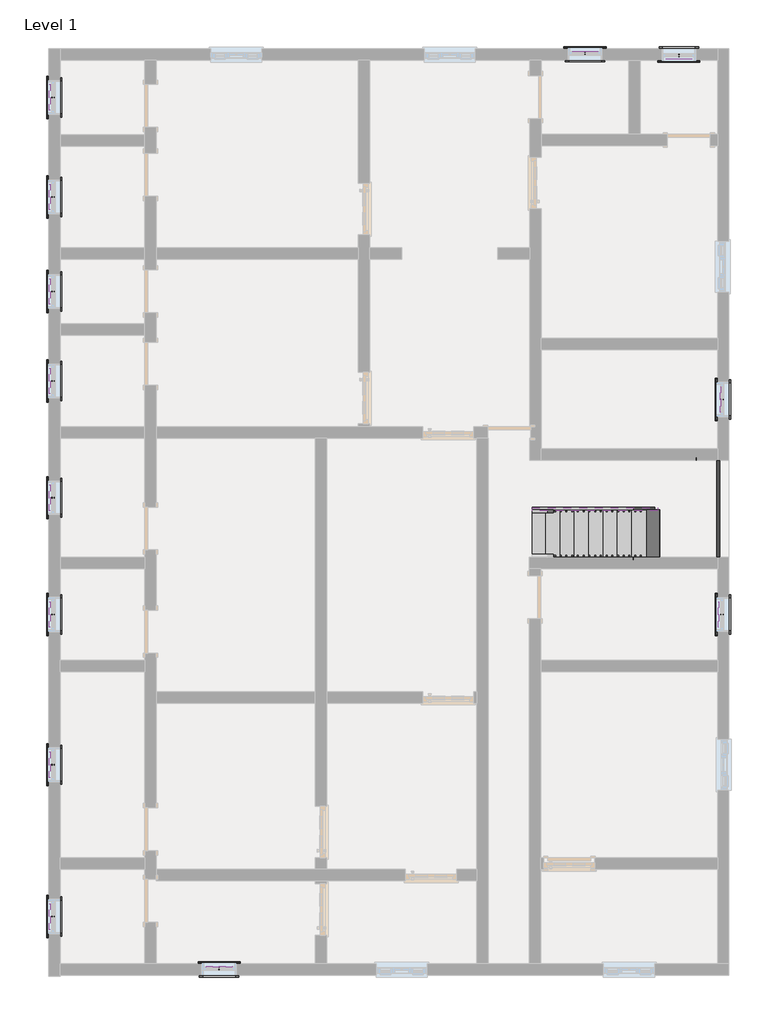
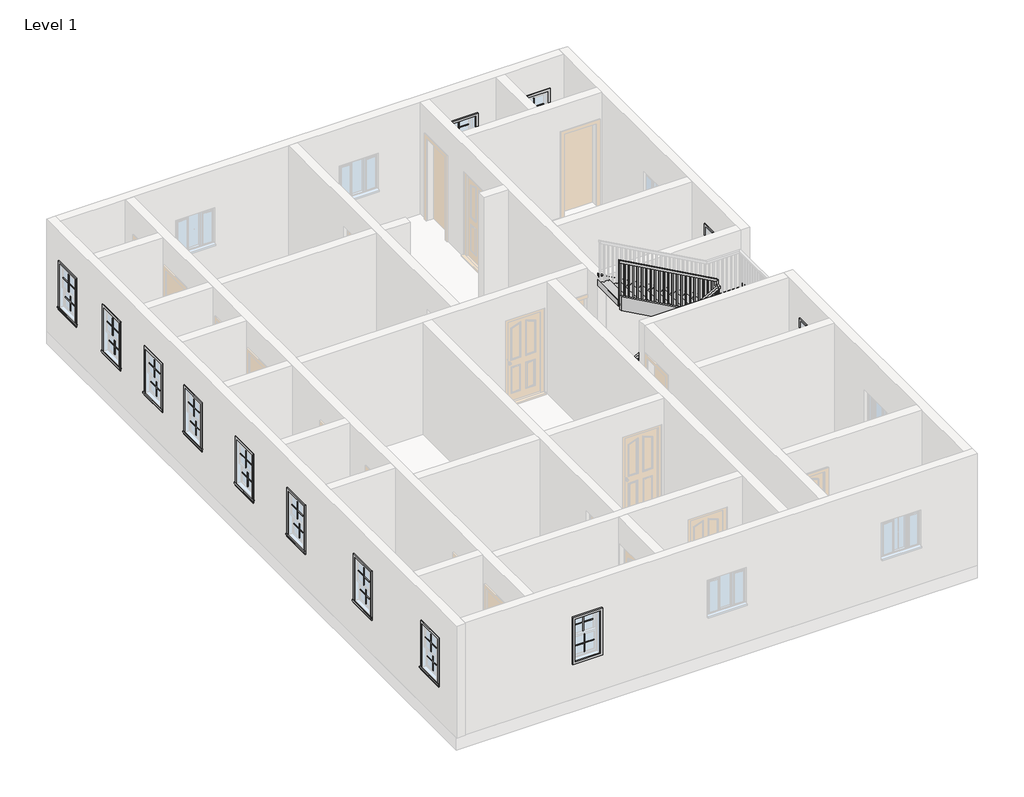
# One storey, part 3 of 3: 52 proxies, 5 members, 1 railing, 1 stair flight.
"""IFC4 building model written with IfcOpenShell, lengths in millimetres."""

from ifc_helpers import new_model, si_unit, frame, origin, place, context, project, spatial, polyline, outline, extrude, faceted_brep, transform, mapped, element, save
from components import muntin_pattern_2x2_muntin_pattern_2x2_eba6c5fb, trim_window_exterior_flat_with_sill_278e6a94, trim_window_interior_flat_picture_frame_e9fd5f45, stair_flight_18d05731

model = new_model("IFC4")

# Units and contexts
model_context = context("Model", 3, world=origin())
ifc_project = project(units=[si_unit("LENGTHUNIT", "METRE", prefix="MILLI")], contexts=[model_context])

# Site, building, storey
site = spatial("IfcSite", under=ifc_project)
building = spatial("IfcBuilding", under=site)
storey = spatial("IfcBuildingStorey", under=building, Name="Level 1", Elevation=0.0)

# Proxies
placement = place(None, origin())
muntin_pattern_2x2_muntin_pattern_2x2_shape = muntin_pattern_2x2_muntin_pattern_2x2_eba6c5fb(model_context)
element("IfcBuildingElementProxy", 1, Name="Muntin Pattern_2x2 : Muntin Pattern_2x2", ObjectType="Muntin Pattern_2x2 : Muntin Pattern_2x2", at=placement, inside=storey, context=model_context, shape_type="MappedRepresentation", body=[
    mapped(muntin_pattern_2x2_muntin_pattern_2x2_shape, transform((-10440.7626145, 6547.3404944, 1470.025), x_axis=(0.0, 1.0, 0.0), y_axis=(-1.0, 0.0, 0.0), z_axis=(0.0, 0.0, 1.0))),
])
element("IfcBuildingElementProxy", 2, Name="Muntin Pattern_2x2 : Muntin Pattern_2x2", ObjectType="Muntin Pattern_2x2 : Muntin Pattern_2x2", at=placement, inside=storey, context=model_context, shape_type="MappedRepresentation", body=[
    mapped(muntin_pattern_2x2_muntin_pattern_2x2_shape, transform((-10396.3126145, 6547.3404944, 990.6), x_axis=(0.0, 1.0, 0.0), y_axis=(-1.0, 0.0, 0.0), z_axis=(0.0, 0.0, 1.0))),
])
element("IfcBuildingElementProxy", 3, Name="Muntin Pattern_2x2 : Muntin Pattern_2x2", ObjectType="Muntin Pattern_2x2 : Muntin Pattern_2x2", at=placement, inside=storey, context=model_context, shape_type="MappedRepresentation", body=[
    mapped(muntin_pattern_2x2_muntin_pattern_2x2_shape, transform((-10440.7626145, 4782.0404944, 1470.025), x_axis=(0.0, 1.0, 0.0), y_axis=(-1.0, 0.0, 0.0), z_axis=(0.0, 0.0, 1.0))),
])
element("IfcBuildingElementProxy", 4, Name="Muntin Pattern_2x2 : Muntin Pattern_2x2", ObjectType="Muntin Pattern_2x2 : Muntin Pattern_2x2", at=placement, inside=storey, context=model_context, shape_type="MappedRepresentation", body=[
    mapped(muntin_pattern_2x2_muntin_pattern_2x2_shape, transform((-10396.3126145, 4782.0404944, 990.6), x_axis=(0.0, 1.0, 0.0), y_axis=(-1.0, 0.0, 0.0), z_axis=(0.0, 0.0, 1.0))),
])
element("IfcBuildingElementProxy", 5, Name="Muntin Pattern_2x2 : Muntin Pattern_2x2", ObjectType="Muntin Pattern_2x2 : Muntin Pattern_2x2", at=placement, inside=storey, context=model_context, shape_type="MappedRepresentation", body=[
    mapped(muntin_pattern_2x2_muntin_pattern_2x2_shape, transform((-10440.7626145, 3105.6404944, 1470.025), x_axis=(0.0, 1.0, 0.0), y_axis=(-1.0, 0.0, 0.0), z_axis=(0.0, 0.0, 1.0))),
])
element("IfcBuildingElementProxy", 6, Name="Muntin Pattern_2x2 : Muntin Pattern_2x2", ObjectType="Muntin Pattern_2x2 : Muntin Pattern_2x2", at=placement, inside=storey, context=model_context, shape_type="MappedRepresentation", body=[
    mapped(muntin_pattern_2x2_muntin_pattern_2x2_shape, transform((-10396.3126145, 3105.6404944, 990.6), x_axis=(0.0, 1.0, 0.0), y_axis=(-1.0, 0.0, 0.0), z_axis=(0.0, 0.0, 1.0))),
])
element("IfcBuildingElementProxy", 7, Name="Muntin Pattern_2x2 : Muntin Pattern_2x2", ObjectType="Muntin Pattern_2x2 : Muntin Pattern_2x2", at=placement, inside=storey, context=model_context, shape_type="MappedRepresentation", body=[
    mapped(muntin_pattern_2x2_muntin_pattern_2x2_shape, transform((-10440.7626145, 1518.1404944, 1470.025), x_axis=(0.0, 1.0, 0.0), y_axis=(-1.0, 0.0, 0.0), z_axis=(0.0, 0.0, 1.0))),
])
element("IfcBuildingElementProxy", 8, Name="Muntin Pattern_2x2 : Muntin Pattern_2x2", ObjectType="Muntin Pattern_2x2 : Muntin Pattern_2x2", at=placement, inside=storey, context=model_context, shape_type="MappedRepresentation", body=[
    mapped(muntin_pattern_2x2_muntin_pattern_2x2_shape, transform((-10396.3126145, 1518.1404944, 990.6), x_axis=(0.0, 1.0, 0.0), y_axis=(-1.0, 0.0, 0.0), z_axis=(0.0, 0.0, 1.0))),
])
element("IfcBuildingElementProxy", 9, Name="Muntin Pattern_2x2 : Muntin Pattern_2x2", ObjectType="Muntin Pattern_2x2 : Muntin Pattern_2x2", at=placement, inside=storey, context=model_context, shape_type="MappedRepresentation", body=[
    mapped(muntin_pattern_2x2_muntin_pattern_2x2_shape, transform((-10440.7626145, -551.9595056, 1470.025), x_axis=(0.0, 1.0, 0.0), y_axis=(-1.0, 0.0, 0.0), z_axis=(0.0, 0.0, 1.0))),
])
element("IfcBuildingElementProxy", 10, Name="Muntin Pattern_2x2 : Muntin Pattern_2x2", ObjectType="Muntin Pattern_2x2 : Muntin Pattern_2x2", at=placement, inside=storey, context=model_context, shape_type="MappedRepresentation", body=[
    mapped(muntin_pattern_2x2_muntin_pattern_2x2_shape, transform((-10396.3126145, -551.9595056, 990.6), x_axis=(0.0, 1.0, 0.0), y_axis=(-1.0, 0.0, 0.0), z_axis=(0.0, 0.0, 1.0))),
])
element("IfcBuildingElementProxy", 11, Name="Muntin Pattern_2x2 : Muntin Pattern_2x2", ObjectType="Muntin Pattern_2x2 : Muntin Pattern_2x2", at=placement, inside=storey, context=model_context, shape_type="MappedRepresentation", body=[
    mapped(muntin_pattern_2x2_muntin_pattern_2x2_shape, transform((-10440.7626145, -2622.0595056, 1470.025), x_axis=(0.0, 1.0, 0.0), y_axis=(-1.0, 0.0, 0.0), z_axis=(0.0, 0.0, 1.0))),
])
element("IfcBuildingElementProxy", 12, Name="Muntin Pattern_2x2 : Muntin Pattern_2x2", ObjectType="Muntin Pattern_2x2 : Muntin Pattern_2x2", at=placement, inside=storey, context=model_context, shape_type="MappedRepresentation", body=[
    mapped(muntin_pattern_2x2_muntin_pattern_2x2_shape, transform((-10396.3126145, -2622.0595056, 990.6), x_axis=(0.0, 1.0, 0.0), y_axis=(-1.0, 0.0, 0.0), z_axis=(0.0, 0.0, 1.0))),
])
element("IfcBuildingElementProxy", 13, Name="Muntin Pattern_2x2 : Muntin Pattern_2x2", ObjectType="Muntin Pattern_2x2 : Muntin Pattern_2x2", at=placement, inside=storey, context=model_context, shape_type="MappedRepresentation", body=[
    mapped(muntin_pattern_2x2_muntin_pattern_2x2_shape, transform((-10440.7626145, -5289.0595056, 1470.025), x_axis=(0.0, 1.0, 0.0), y_axis=(-1.0, 0.0, 0.0), z_axis=(0.0, 0.0, 1.0))),
])
element("IfcBuildingElementProxy", 14, Name="Muntin Pattern_2x2 : Muntin Pattern_2x2", ObjectType="Muntin Pattern_2x2 : Muntin Pattern_2x2", at=placement, inside=storey, context=model_context, shape_type="MappedRepresentation", body=[
    mapped(muntin_pattern_2x2_muntin_pattern_2x2_shape, transform((-10396.3126145, -5289.0595056, 990.6), x_axis=(0.0, 1.0, 0.0), y_axis=(-1.0, 0.0, 0.0), z_axis=(0.0, 0.0, 1.0))),
])
element("IfcBuildingElementProxy", 15, Name="Muntin Pattern_2x2 : Muntin Pattern_2x2", ObjectType="Muntin Pattern_2x2 : Muntin Pattern_2x2", at=placement, inside=storey, context=model_context, shape_type="MappedRepresentation", body=[
    mapped(muntin_pattern_2x2_muntin_pattern_2x2_shape, transform((-10440.7626145, -7981.4595056, 1470.025), x_axis=(0.0, 1.0, 0.0), y_axis=(-1.0, 0.0, 0.0), z_axis=(0.0, 0.0, 1.0))),
])
element("IfcBuildingElementProxy", 16, Name="Muntin Pattern_2x2 : Muntin Pattern_2x2", ObjectType="Muntin Pattern_2x2 : Muntin Pattern_2x2", at=placement, inside=storey, context=model_context, shape_type="MappedRepresentation", body=[
    mapped(muntin_pattern_2x2_muntin_pattern_2x2_shape, transform((-10396.3126145, -7981.4595056, 990.6), x_axis=(0.0, 1.0, 0.0), y_axis=(-1.0, 0.0, 0.0), z_axis=(0.0, 0.0, 1.0))),
])
element("IfcBuildingElementProxy", 17, Name="Muntin Pattern_2x2 : Muntin Pattern_2x2", ObjectType="Muntin Pattern_2x2 : Muntin Pattern_2x2", at=placement, inside=storey, context=model_context, shape_type="MappedRepresentation", body=[
    mapped(muntin_pattern_2x2_muntin_pattern_2x2_shape, transform((-7453.0876145, -8854.5845056, 1470.025), x_axis=(1.0, 0.0, 0.0), y_axis=(0.0, 1.0, 0.0), z_axis=(0.0, 0.0, 1.0))),
])
element("IfcBuildingElementProxy", 18, Name="Muntin Pattern_2x2 : Muntin Pattern_2x2", ObjectType="Muntin Pattern_2x2 : Muntin Pattern_2x2", at=placement, inside=storey, context=model_context, shape_type="MappedRepresentation", body=[
    mapped(muntin_pattern_2x2_muntin_pattern_2x2_shape, transform((-7453.0876145, -8899.0345056, 990.6), x_axis=(1.0, 0.0, 0.0), y_axis=(0.0, 1.0, 0.0), z_axis=(0.0, 0.0, 1.0))),
])
element("IfcBuildingElementProxy", 19, Name="Muntin Pattern_2x2 : Muntin Pattern_2x2", ObjectType="Muntin Pattern_2x2 : Muntin Pattern_2x2", at=placement, inside=storey, context=model_context, shape_type="MappedRepresentation", body=[
    mapped(muntin_pattern_2x2_muntin_pattern_2x2_shape, transform((1421.0373855, -2622.0595056, 1470.025), x_axis=(0.0, 1.0, 0.0), y_axis=(-1.0, 0.0, 0.0), z_axis=(0.0, 0.0, 1.0))),
])
element("IfcBuildingElementProxy", 20, Name="Muntin Pattern_2x2 : Muntin Pattern_2x2", ObjectType="Muntin Pattern_2x2 : Muntin Pattern_2x2", at=placement, inside=storey, context=model_context, shape_type="MappedRepresentation", body=[
    mapped(muntin_pattern_2x2_muntin_pattern_2x2_shape, transform((1465.4873855, -2622.0595056, 990.6), x_axis=(0.0, 1.0, 0.0), y_axis=(-1.0, 0.0, 0.0), z_axis=(0.0, 0.0, 1.0))),
])
element("IfcBuildingElementProxy", 21, Name="Muntin Pattern_2x2 : Muntin Pattern_2x2", ObjectType="Muntin Pattern_2x2 : Muntin Pattern_2x2", at=placement, inside=storey, context=model_context, shape_type="MappedRepresentation", body=[
    mapped(muntin_pattern_2x2_muntin_pattern_2x2_shape, transform((1421.0373855, 1190.4645364, 1470.025), x_axis=(0.0, 1.0, 0.0), y_axis=(-1.0, 0.0, 0.0), z_axis=(0.0, 0.0, 1.0))),
])
element("IfcBuildingElementProxy", 22, Name="Muntin Pattern_2x2 : Muntin Pattern_2x2", ObjectType="Muntin Pattern_2x2 : Muntin Pattern_2x2", at=placement, inside=storey, context=model_context, shape_type="MappedRepresentation", body=[
    mapped(muntin_pattern_2x2_muntin_pattern_2x2_shape, transform((1465.4873855, 1190.4645364, 990.6), x_axis=(0.0, 1.0, 0.0), y_axis=(-1.0, 0.0, 0.0), z_axis=(0.0, 0.0, 1.0))),
])
element("IfcBuildingElementProxy", 23, Name="Muntin Pattern_2x2 : Muntin Pattern_2x2", ObjectType="Muntin Pattern_2x2 : Muntin Pattern_2x2", at=placement, inside=storey, context=model_context, shape_type="MappedRepresentation", body=[
    mapped(muntin_pattern_2x2_muntin_pattern_2x2_shape, transform((700.3123855, 7242.6654944, 1470.025), x_axis=(-1.0, 0.0, 0.0), y_axis=(0.0, -1.0, 0.0), z_axis=(0.0, 0.0, 1.0))),
])
element("IfcBuildingElementProxy", 24, Name="Muntin Pattern_2x2 : Muntin Pattern_2x2", ObjectType="Muntin Pattern_2x2 : Muntin Pattern_2x2", at=placement, inside=storey, context=model_context, shape_type="MappedRepresentation", body=[
    mapped(muntin_pattern_2x2_muntin_pattern_2x2_shape, transform((700.3123855, 7287.1154944, 990.6), x_axis=(-1.0, 0.0, 0.0), y_axis=(0.0, -1.0, 0.0), z_axis=(0.0, 0.0, 1.0))),
])
element("IfcBuildingElementProxy", 25, Name="Muntin Pattern_2x2 : Muntin Pattern_2x2", ObjectType="Muntin Pattern_2x2 : Muntin Pattern_2x2", at=placement, inside=storey, context=model_context, shape_type="MappedRepresentation", body=[
    mapped(muntin_pattern_2x2_muntin_pattern_2x2_shape, transform((-963.3876145, 7376.0154944, 1470.025), x_axis=(1.0, 0.0, 0.0), y_axis=(0.0, 1.0, 0.0), z_axis=(0.0, 0.0, 1.0))),
])
element("IfcBuildingElementProxy", 26, Name="Muntin Pattern_2x2 : Muntin Pattern_2x2", ObjectType="Muntin Pattern_2x2 : Muntin Pattern_2x2", at=placement, inside=storey, context=model_context, shape_type="MappedRepresentation", body=[
    mapped(muntin_pattern_2x2_muntin_pattern_2x2_shape, transform((-963.3876145, 7331.5654944, 990.6), x_axis=(1.0, 0.0, 0.0), y_axis=(0.0, 1.0, 0.0), z_axis=(0.0, 0.0, 1.0))),
])
trim_window_exterior_flat_with_sill_shape = trim_window_exterior_flat_with_sill_278e6a94(model_context)
element("IfcBuildingElementProxy", 27, Name="Trim-Window-Exterior-Flat : with Sill", ObjectType="Trim-Window-Exterior-Flat : with Sill", at=placement, inside=storey, context=model_context, shape_type="MappedRepresentation", body=[
    mapped(trim_window_exterior_flat_with_sill_shape, transform((-10475.6876145, 6547.3404944, 1981.2), x_axis=(0.0, -1.0, 0.0), y_axis=(0.0, 0.0, 1.0), z_axis=(-1.0, 0.0, 0.0))),
])
element("IfcBuildingElementProxy", 28, Name="Trim-Window-Exterior-Flat : with Sill", ObjectType="Trim-Window-Exterior-Flat : with Sill", at=placement, inside=storey, context=model_context, shape_type="MappedRepresentation", body=[
    mapped(trim_window_exterior_flat_with_sill_shape, transform((-10475.6876145, 4782.0404944, 1981.2), x_axis=(0.0, -1.0, 0.0), y_axis=(0.0, 0.0, 1.0), z_axis=(-1.0, 0.0, 0.0))),
])
element("IfcBuildingElementProxy", 29, Name="Trim-Window-Exterior-Flat : with Sill", ObjectType="Trim-Window-Exterior-Flat : with Sill", at=placement, inside=storey, context=model_context, shape_type="MappedRepresentation", body=[
    mapped(trim_window_exterior_flat_with_sill_shape, transform((-10475.6876145, 3105.6404944, 1981.2), x_axis=(0.0, -1.0, 0.0), y_axis=(0.0, 0.0, 1.0), z_axis=(-1.0, 0.0, 0.0))),
])
element("IfcBuildingElementProxy", 30, Name="Trim-Window-Exterior-Flat : with Sill", ObjectType="Trim-Window-Exterior-Flat : with Sill", at=placement, inside=storey, context=model_context, shape_type="MappedRepresentation", body=[
    mapped(trim_window_exterior_flat_with_sill_shape, transform((-10475.6876145, 1518.1404944, 1981.2), x_axis=(0.0, -1.0, 0.0), y_axis=(0.0, 0.0, 1.0), z_axis=(-1.0, 0.0, 0.0))),
])
element("IfcBuildingElementProxy", 31, Name="Trim-Window-Exterior-Flat : with Sill", ObjectType="Trim-Window-Exterior-Flat : with Sill", at=placement, inside=storey, context=model_context, shape_type="MappedRepresentation", body=[
    mapped(trim_window_exterior_flat_with_sill_shape, transform((-10475.6876145, -551.9595056, 1981.2), x_axis=(0.0, -1.0, 0.0), y_axis=(0.0, 0.0, 1.0), z_axis=(-1.0, 0.0, 0.0))),
])
element("IfcBuildingElementProxy", 32, Name="Trim-Window-Exterior-Flat : with Sill", ObjectType="Trim-Window-Exterior-Flat : with Sill", at=placement, inside=storey, context=model_context, shape_type="MappedRepresentation", body=[
    mapped(trim_window_exterior_flat_with_sill_shape, transform((-10475.6876145, -2622.0595056, 1981.2), x_axis=(0.0, -1.0, 0.0), y_axis=(0.0, 0.0, 1.0), z_axis=(-1.0, 0.0, 0.0))),
])
element("IfcBuildingElementProxy", 33, Name="Trim-Window-Exterior-Flat : with Sill", ObjectType="Trim-Window-Exterior-Flat : with Sill", at=placement, inside=storey, context=model_context, shape_type="MappedRepresentation", body=[
    mapped(trim_window_exterior_flat_with_sill_shape, transform((-10475.6876145, -5289.0595056, 1981.2), x_axis=(0.0, -1.0, 0.0), y_axis=(0.0, 0.0, 1.0), z_axis=(-1.0, 0.0, 0.0))),
])
element("IfcBuildingElementProxy", 34, Name="Trim-Window-Exterior-Flat : with Sill", ObjectType="Trim-Window-Exterior-Flat : with Sill", at=placement, inside=storey, context=model_context, shape_type="MappedRepresentation", body=[
    mapped(trim_window_exterior_flat_with_sill_shape, transform((-10475.6876145, -7981.4595056, 1981.2), x_axis=(0.0, -1.0, 0.0), y_axis=(0.0, 0.0, 1.0), z_axis=(-1.0, 0.0, 0.0))),
])
element("IfcBuildingElementProxy", 35, Name="Trim-Window-Exterior-Flat : with Sill", ObjectType="Trim-Window-Exterior-Flat : with Sill", at=placement, inside=storey, context=model_context, shape_type="MappedRepresentation", body=[
    mapped(trim_window_exterior_flat_with_sill_shape, transform((-7453.0876145, -8819.6595056, 1981.2), x_axis=(-1.0, 0.0, 0.0), y_axis=(0.0, 0.0, 1.0), z_axis=(0.0, 1.0, 0.0))),
])
element("IfcBuildingElementProxy", 36, Name="Trim-Window-Exterior-Flat : with Sill", ObjectType="Trim-Window-Exterior-Flat : with Sill", at=placement, inside=storey, context=model_context, shape_type="MappedRepresentation", body=[
    mapped(trim_window_exterior_flat_with_sill_shape, transform((1386.1123855, -2622.0595056, 1981.2), x_axis=(0.0, -1.0, 0.0), y_axis=(0.0, 0.0, 1.0), z_axis=(-1.0, 0.0, 0.0))),
])
element("IfcBuildingElementProxy", 37, Name="Trim-Window-Exterior-Flat : with Sill", ObjectType="Trim-Window-Exterior-Flat : with Sill", at=placement, inside=storey, context=model_context, shape_type="MappedRepresentation", body=[
    mapped(trim_window_exterior_flat_with_sill_shape, transform((1386.1123855, 1190.4645364, 1981.2), x_axis=(0.0, -1.0, 0.0), y_axis=(0.0, 0.0, 1.0), z_axis=(-1.0, 0.0, 0.0))),
])
element("IfcBuildingElementProxy", 38, Name="Trim-Window-Exterior-Flat : with Sill", ObjectType="Trim-Window-Exterior-Flat : with Sill", at=placement, inside=storey, context=model_context, shape_type="MappedRepresentation", body=[
    mapped(trim_window_exterior_flat_with_sill_shape, transform((700.3123855, 7207.7404944, 1981.2), x_axis=(1.0, 0.0, 0.0), y_axis=(0.0, 0.0, 1.0), z_axis=(0.0, -1.0, 0.0))),
])
element("IfcBuildingElementProxy", 39, Name="Trim-Window-Exterior-Flat : with Sill", ObjectType="Trim-Window-Exterior-Flat : with Sill", at=placement, inside=storey, context=model_context, shape_type="MappedRepresentation", body=[
    mapped(trim_window_exterior_flat_with_sill_shape, transform((-963.3876145, 7410.9404944, 1981.2), x_axis=(-1.0, 0.0, 0.0), y_axis=(0.0, 0.0, 1.0), z_axis=(0.0, 1.0, 0.0))),
])
trim_window_interior_flat_picture_frame_shape = trim_window_interior_flat_picture_frame_e9fd5f45(model_context)
element("IfcBuildingElementProxy", 40, Name="Trim-Window-Interior-Flat : Picture Frame", ObjectType="Trim-Window-Interior-Flat : Picture Frame", at=placement, inside=storey, context=model_context, shape_type="MappedRepresentation", body=[
    mapped(trim_window_interior_flat_picture_frame_shape, transform((-10272.4876145, 6547.3404944, 1981.2), x_axis=(0.0, 1.0, 0.0), y_axis=(0.0, 0.0, 1.0), z_axis=(1.0, 0.0, 0.0))),
])
element("IfcBuildingElementProxy", 41, Name="Trim-Window-Interior-Flat : Picture Frame", ObjectType="Trim-Window-Interior-Flat : Picture Frame", at=placement, inside=storey, context=model_context, shape_type="MappedRepresentation", body=[
    mapped(trim_window_interior_flat_picture_frame_shape, transform((-10272.4876145, 4782.0404944, 1981.2), x_axis=(0.0, 1.0, 0.0), y_axis=(0.0, 0.0, 1.0), z_axis=(1.0, 0.0, 0.0))),
])
element("IfcBuildingElementProxy", 42, Name="Trim-Window-Interior-Flat : Picture Frame", ObjectType="Trim-Window-Interior-Flat : Picture Frame", at=placement, inside=storey, context=model_context, shape_type="MappedRepresentation", body=[
    mapped(trim_window_interior_flat_picture_frame_shape, transform((-10272.4876145, 3105.6404944, 1981.2), x_axis=(0.0, 1.0, 0.0), y_axis=(0.0, 0.0, 1.0), z_axis=(1.0, 0.0, 0.0))),
])
element("IfcBuildingElementProxy", 43, Name="Trim-Window-Interior-Flat : Picture Frame", ObjectType="Trim-Window-Interior-Flat : Picture Frame", at=placement, inside=storey, context=model_context, shape_type="MappedRepresentation", body=[
    mapped(trim_window_interior_flat_picture_frame_shape, transform((-10272.4876145, 1518.1404944, 1981.2), x_axis=(0.0, 1.0, 0.0), y_axis=(0.0, 0.0, 1.0), z_axis=(1.0, 0.0, 0.0))),
])
element("IfcBuildingElementProxy", 44, Name="Trim-Window-Interior-Flat : Picture Frame", ObjectType="Trim-Window-Interior-Flat : Picture Frame", at=placement, inside=storey, context=model_context, shape_type="MappedRepresentation", body=[
    mapped(trim_window_interior_flat_picture_frame_shape, transform((-10272.4876145, -551.9595056, 1981.2), x_axis=(0.0, 1.0, 0.0), y_axis=(0.0, 0.0, 1.0), z_axis=(1.0, 0.0, 0.0))),
])
element("IfcBuildingElementProxy", 45, Name="Trim-Window-Interior-Flat : Picture Frame", ObjectType="Trim-Window-Interior-Flat : Picture Frame", at=placement, inside=storey, context=model_context, shape_type="MappedRepresentation", body=[
    mapped(trim_window_interior_flat_picture_frame_shape, transform((-10272.4876145, -2622.0595056, 1981.2), x_axis=(0.0, 1.0, 0.0), y_axis=(0.0, 0.0, 1.0), z_axis=(1.0, 0.0, 0.0))),
])
element("IfcBuildingElementProxy", 46, Name="Trim-Window-Interior-Flat : Picture Frame", ObjectType="Trim-Window-Interior-Flat : Picture Frame", at=placement, inside=storey, context=model_context, shape_type="MappedRepresentation", body=[
    mapped(trim_window_interior_flat_picture_frame_shape, transform((-10272.4876145, -5289.0595056, 1981.2), x_axis=(0.0, 1.0, 0.0), y_axis=(0.0, 0.0, 1.0), z_axis=(1.0, 0.0, 0.0))),
])
element("IfcBuildingElementProxy", 47, Name="Trim-Window-Interior-Flat : Picture Frame", ObjectType="Trim-Window-Interior-Flat : Picture Frame", at=placement, inside=storey, context=model_context, shape_type="MappedRepresentation", body=[
    mapped(trim_window_interior_flat_picture_frame_shape, transform((-10272.4876145, -7981.4595056, 1981.2), x_axis=(0.0, 1.0, 0.0), y_axis=(0.0, 0.0, 1.0), z_axis=(1.0, 0.0, 0.0))),
])
element("IfcBuildingElementProxy", 48, Name="Trim-Window-Interior-Flat : Picture Frame", ObjectType="Trim-Window-Interior-Flat : Picture Frame", at=placement, inside=storey, context=model_context, shape_type="MappedRepresentation", body=[
    mapped(trim_window_interior_flat_picture_frame_shape, transform((-7453.0876145, -9022.8595056, 1981.2), x_axis=(1.0, 0.0, 0.0), y_axis=(0.0, 0.0, 1.0), z_axis=(0.0, -1.0, 0.0))),
])
element("IfcBuildingElementProxy", 49, Name="Trim-Window-Interior-Flat : Picture Frame", ObjectType="Trim-Window-Interior-Flat : Picture Frame", at=placement, inside=storey, context=model_context, shape_type="MappedRepresentation", body=[
    mapped(trim_window_interior_flat_picture_frame_shape, transform((1589.3123855, -2622.0595056, 1981.2), x_axis=(0.0, 1.0, 0.0), y_axis=(0.0, 0.0, 1.0), z_axis=(1.0, 0.0, 0.0))),
])
element("IfcBuildingElementProxy", 50, Name="Trim-Window-Interior-Flat : Picture Frame", ObjectType="Trim-Window-Interior-Flat : Picture Frame", at=placement, inside=storey, context=model_context, shape_type="MappedRepresentation", body=[
    mapped(trim_window_interior_flat_picture_frame_shape, transform((1589.3123855, 1190.4645364, 1981.2), x_axis=(0.0, 1.0, 0.0), y_axis=(0.0, 0.0, 1.0), z_axis=(1.0, 0.0, 0.0))),
])
element("IfcBuildingElementProxy", 51, Name="Trim-Window-Interior-Flat : Picture Frame", ObjectType="Trim-Window-Interior-Flat : Picture Frame", at=placement, inside=storey, context=model_context, shape_type="MappedRepresentation", body=[
    mapped(trim_window_interior_flat_picture_frame_shape, transform((700.3123855, 7410.9404944, 1981.2), x_axis=(-1.0, 0.0, 0.0), y_axis=(0.0, 0.0, 1.0), z_axis=(0.0, 1.0, 0.0))),
])
element("IfcBuildingElementProxy", 52, Name="Trim-Window-Interior-Flat : Picture Frame", ObjectType="Trim-Window-Interior-Flat : Picture Frame", at=placement, inside=storey, context=model_context, shape_type="MappedRepresentation", body=[
    mapped(trim_window_interior_flat_picture_frame_shape, transform((-963.3876145, 7207.7404944, 1981.2), x_axis=(1.0, 0.0, 0.0), y_axis=(0.0, 0.0, 1.0), z_axis=(0.0, -1.0, 0.0))),
])

# Members
element("IfcMember", 53, ObjectType="Stringer - 2\" Width", at=placement, inside=storey, context=model_context, shape_type="SweptSolid", body=[
    extrude(outline(polyline([(210.6757607, -1903.1876145), (0.0, -1903.1876145), (0.0, -1654.2050647), (1065.4963497, 274.6830625), (1413.7073019, 274.6830625), (210.6757607, -1903.1876145)])), frame((0.0, -767.8595056, 0.0), z_axis=(0.0, 1.0, 0.0), x_axis=(0.0, 0.0, 1.0)), (0.0, 0.0, 1.0), 50.8),
])
element("IfcMember", 54, ObjectType="Stringer - 2\" Width", at=placement, inside=storey, context=model_context, shape_type="SweptSolid", body=[
    extrude(outline(polyline([(1230.7177047, 325.4830625), (1578.928657, 325.4830625), (2810.0215532, -1903.1876145), (2461.8106009, -1903.1876145), (1230.7177047, 325.4830625)])), frame((0.0, -780.5595056, 0.0), z_axis=(0.0, 1.0, 0.0), x_axis=(0.0, 0.0, 1.0)), (0.0, 0.0, 1.0), 50.8),
])
element("IfcMember", 55, ObjectType="Stringer - 2\" Width", at=placement, inside=storey, context=model_context, shape_type="SweptSolid", body=[
    extrude(outline(polyline([(210.6757607, -1903.1876145), (0.0, -1903.1876145), (0.0, -1654.2050647), (1447.8, 966.7745674), (1447.8, 336.4017165), (210.6757607, -1903.1876145)])), frame((0.0, -1656.8595056, 0.0), z_axis=(0.0, 1.0, 0.0), x_axis=(0.0, 0.0, 1.0)), (0.0, 0.0, 1.0), 50.8),
])
element("IfcMember", 56, ObjectType="Stringer - 2\" Width", at=placement, inside=storey, context=model_context, shape_type="SweptSolid", body=[
    extrude(outline(polyline([(1424.2123855, -1656.8595056), (1373.4123855, -1656.8595056), (1373.4123855, 108.4404944), (1424.2123855, 108.4404944), (1424.2123855, -1656.8595056)])), frame((0.0, 0.0, 1143.0), z_axis=(0.0, 0.0, 1.0), x_axis=(1.0, 0.0, 0.0)), (0.0, 0.0, 1.0), 304.8),
])
element("IfcMember", 57, ObjectType="Stringer - 2\" Width", at=placement, inside=storey, context=model_context, shape_type="SweptSolid", body=[
    extrude(outline(polyline([(1143.0, 1114.6529278), (2810.0215532, -1903.1876145), (2461.8106009, -1903.1876145), (1143.0, 484.2800769), (1143.0, 1114.6529278)])), frame((0.0, 108.4404944, 0.0), z_axis=(0.0, 1.0, 0.0), x_axis=(0.0, 0.0, 1.0)), (0.0, 0.0, 1.0), 50.8),
])

# Railing
element("IfcRailing", 58, ObjectType="Handrail - Rectangular", at=placement, inside=storey, context=model_context, shape_type="SolidModel", body=[
    faceted_brep([(-1903.1876145, -767.8595056, 1051.56), (-1903.1876145, -767.8595056, 993.4879132), (-1903.1876145, -818.6595056, 993.4879132), (-1903.1876145, -818.6595056, 1051.56), (325.4830625, -767.8595056, 2286.0), (325.4830625, -818.6595056, 2286.0), (325.4830625, -818.6595056, 2227.9279132), (325.4830625, -767.8595056, 2227.9279132)], [[[0, 1, 2, 3]], [[4, 5, 6, 7]], [[1, 0, 4, 7]], [[2, 1, 7, 6]], [[3, 2, 6, 5]], [[0, 3, 5, 4]]]),
    faceted_brep([(325.4830625, -818.6595056, 2286.0), (325.4830625, -818.6595056, 2235.2), (376.2830625, -818.6595056, 2235.2), (376.2830625, -818.6595056, 2286.0), (325.4830625, -729.7595056, 2286.0), (376.2830625, -729.7595056, 2286.0), (376.2830625, -678.9595056, 2235.2), (325.4830625, -678.9595056, 2235.2)], [[[0, 1, 2, 3]], [[4, 5, 6, 7]], [[1, 0, 4, 7]], [[2, 1, 7, 6]], [[3, 2, 6, 5]], [[0, 3, 5, 4]]]),
    faceted_brep([(325.4830625, -729.7595056, 2286.0), (325.4830625, -678.9595056, 2235.2), (376.2830625, -678.9595056, 2235.2), (376.2830625, -729.7595056, 2286.0), (325.4830625, -729.7595056, 2365.0879132), (376.2830625, -729.7595056, 2395.0223516), (376.2830625, -678.9595056, 2395.0223516), (325.4830625, -678.9595056, 2365.0879132)], [[[0, 1, 2, 3]], [[4, 5, 6, 7]], [[1, 0, 4, 7]], [[2, 1, 7, 6]], [[3, 2, 6, 5]], [[0, 3, 5, 4]]]),
    faceted_brep([(376.2830625, -729.7595056, 2395.0223516), (325.4830625, -729.7595056, 2365.0879132), (325.4830625, -678.9595056, 2365.0879132), (376.2830625, -678.9595056, 2395.0223516), (-1903.1876145, -729.7595056, 3657.6), (-1903.1876145, -678.9595056, 3657.6), (-1903.1876145, -678.9595056, 3599.5279132), (-1903.1876145, -729.7595056, 3599.5279132)], [[[0, 1, 2, 3]], [[4, 5, 6, 7]], [[1, 0, 4, 7]], [[2, 1, 7, 6]], [[3, 2, 6, 5]], [[0, 3, 5, 4]]]),
    extrude(outline(polyline([(3594.3072849, -1893.8419375), (2606.04, -1893.8419375), (2606.04, -1874.7919375), (3583.7556667, -1874.7919375), (3594.3072849, -1893.8419375)])), frame((0.0, -713.8845056, 0.0), z_axis=(0.0, 1.0, 0.0), x_axis=(0.0, 0.0, 1.0)), (0.0, 0.0, 1.0), 19.05),
    extrude(outline(polyline([(3538.031988, -1792.2419375), (2606.04, -1792.2419375), (2606.04, -1773.1919375), (3527.4803699, -1773.1919375), (3538.031988, -1792.2419375)])), frame((0.0, -713.8845056, 0.0), z_axis=(0.0, 1.0, 0.0), x_axis=(0.0, 0.0, 1.0)), (0.0, 0.0, 1.0), 19.05),
    extrude(outline(polyline([(3481.7125466, -1690.6419375), (2606.04, -1690.6419375), (2606.04, -1671.5919375), (3471.1609284, -1671.5919375), (3481.7125466, -1690.6419375)])), frame((0.0, -713.8845056, 0.0), z_axis=(0.0, 1.0, 0.0), x_axis=(0.0, 0.0, 1.0)), (0.0, 0.0, 1.0), 19.05),
    extrude(outline(polyline([(3425.4813943, -1589.0419375), (2468.88, -1589.0419375), (2468.88, -1569.9919375), (3414.9297761, -1569.9919375), (3425.4813943, -1589.0419375)])), frame((0.0, -713.8845056, 0.0), z_axis=(0.0, 1.0, 0.0), x_axis=(0.0, 0.0, 1.0)), (0.0, 0.0, 1.0), 19.05),
    extrude(outline(polyline([(3369.2060974, -1487.4419375), (2468.88, -1487.4419375), (2468.88, -1468.3919375), (3358.6544792, -1468.3919375), (3369.2060974, -1487.4419375)])), frame((0.0, -713.8845056, 0.0), z_axis=(0.0, 1.0, 0.0), x_axis=(0.0, 0.0, 1.0)), (0.0, 0.0, 1.0), 19.05),
    extrude(outline(polyline([(3312.9308005, -1385.8419375), (2331.72, -1385.8419375), (2331.72, -1366.7919375), (3302.3791823, -1366.7919375), (3312.9308005, -1385.8419375)])), frame((0.0, -713.8845056, 0.0), z_axis=(0.0, 1.0, 0.0), x_axis=(0.0, 0.0, 1.0)), (0.0, 0.0, 1.0), 19.05),
    extrude(outline(polyline([(3256.6555036, -1284.2419375), (2331.72, -1284.2419375), (2331.72, -1265.1919375), (3246.1038855, -1265.1919375), (3256.6555036, -1284.2419375)])), frame((0.0, -713.8845056, 0.0), z_axis=(0.0, 1.0, 0.0), x_axis=(0.0, 0.0, 1.0)), (0.0, 0.0, 1.0), 19.05),
    extrude(outline(polyline([(3200.3802067, -1182.6419375), (2331.72, -1182.6419375), (2331.72, -1163.5919375), (3189.8285886, -1163.5919375), (3200.3802067, -1182.6419375)])), frame((0.0, -713.8845056, 0.0), z_axis=(0.0, 1.0, 0.0), x_axis=(0.0, 0.0, 1.0)), (0.0, 0.0, 1.0), 19.05),
    extrude(outline(polyline([(3144.1049099, -1081.0419375), (2194.56, -1081.0419375), (2194.56, -1061.9919375), (3133.5532917, -1061.9919375), (3144.1049099, -1081.0419375)])), frame((0.0, -713.8845056, 0.0), z_axis=(0.0, 1.0, 0.0), x_axis=(0.0, 0.0, 1.0)), (0.0, 0.0, 1.0), 19.05),
    extrude(outline(polyline([(3087.829613, -979.4419375), (2194.56, -979.4419375), (2194.56, -960.3919375), (3077.2779948, -960.3919375), (3087.829613, -979.4419375)])), frame((0.0, -713.8845056, 0.0), z_axis=(0.0, 1.0, 0.0), x_axis=(0.0, 0.0, 1.0)), (0.0, 0.0, 1.0), 19.05),
    extrude(outline(polyline([(3031.5543161, -877.8419375), (2057.4, -877.8419375), (2057.4, -858.7919375), (3021.0026979, -858.7919375), (3031.5543161, -877.8419375)])), frame((0.0, -713.8845056, 0.0), z_axis=(0.0, 1.0, 0.0), x_axis=(0.0, 0.0, 1.0)), (0.0, 0.0, 1.0), 19.05),
    extrude(outline(polyline([(2975.2790192, -776.2419375), (2057.4, -776.2419375), (2057.4, -757.1919375), (2964.727401, -757.1919375), (2975.2790192, -776.2419375)])), frame((0.0, -713.8845056, 0.0), z_axis=(0.0, 1.0, 0.0), x_axis=(0.0, 0.0, 1.0)), (0.0, 0.0, 1.0), 19.05),
    extrude(outline(polyline([(2919.0478669, -674.6419375), (2057.4, -674.6419375), (2057.4, -655.5919375), (2908.4962488, -655.5919375), (2919.0478669, -674.6419375)])), frame((0.0, -713.8845056, 0.0), z_axis=(0.0, 1.0, 0.0), x_axis=(0.0, 0.0, 1.0)), (0.0, 0.0, 1.0), 19.05),
    extrude(outline(polyline([(2862.77257, -573.0419375), (1920.24, -573.0419375), (1920.24, -553.9919375), (2852.2209519, -553.9919375), (2862.77257, -573.0419375)])), frame((0.0, -713.8845056, 0.0), z_axis=(0.0, 1.0, 0.0), x_axis=(0.0, 0.0, 1.0)), (0.0, 0.0, 1.0), 19.05),
    extrude(outline(polyline([(2806.4972732, -471.4419375), (1920.24, -471.4419375), (1920.24, -452.3919375), (2795.945655, -452.3919375), (2806.4972732, -471.4419375)])), frame((0.0, -713.8845056, 0.0), z_axis=(0.0, 1.0, 0.0), x_axis=(0.0, 0.0, 1.0)), (0.0, 0.0, 1.0), 19.05),
    extrude(outline(polyline([(2750.2219763, -369.8419375), (1783.08, -369.8419375), (1783.08, -350.7919375), (2739.6703581, -350.7919375), (2750.2219763, -369.8419375)])), frame((0.0, -713.8845056, 0.0), z_axis=(0.0, 1.0, 0.0), x_axis=(0.0, 0.0, 1.0)), (0.0, 0.0, 1.0), 19.05),
    extrude(outline(polyline([(2693.9466794, -268.2419375), (1783.08, -268.2419375), (1783.08, -249.1919375), (2683.3950612, -249.1919375), (2693.9466794, -268.2419375)])), frame((0.0, -713.8845056, 0.0), z_axis=(0.0, 1.0, 0.0), x_axis=(0.0, 0.0, 1.0)), (0.0, 0.0, 1.0), 19.05),
    extrude(outline(polyline([(2637.6713825, -166.6419375), (1783.08, -166.6419375), (1783.08, -147.5919375), (2627.1197643, -147.5919375), (2637.6713825, -166.6419375)])), frame((0.0, -713.8845056, 0.0), z_axis=(0.0, 1.0, 0.0), x_axis=(0.0, 0.0, 1.0)), (0.0, 0.0, 1.0), 19.05),
    extrude(outline(polyline([(2581.3960856, -65.0419375), (1645.92, -65.0419375), (1645.92, -45.9919375), (2570.8444675, -45.9919375), (2581.3960856, -65.0419375)])), frame((0.0, -713.8845056, 0.0), z_axis=(0.0, 1.0, 0.0), x_axis=(0.0, 0.0, 1.0)), (0.0, 0.0, 1.0), 19.05),
    extrude(outline(polyline([(2525.1207888, 36.5580625), (1645.92, 36.5580625), (1645.92, 55.6080625), (2514.5691706, 55.6080625), (2525.1207888, 36.5580625)])), frame((0.0, -713.8845056, 0.0), z_axis=(0.0, 1.0, 0.0), x_axis=(0.0, 0.0, 1.0)), (0.0, 0.0, 1.0), 19.05),
    extrude(outline(polyline([(2468.8454919, 138.1580625), (1508.76, 138.1580625), (1508.76, 157.2080625), (2458.2938737, 157.2080625), (2468.8454919, 138.1580625)])), frame((0.0, -713.8845056, 0.0), z_axis=(0.0, 1.0, 0.0), x_axis=(0.0, 0.0, 1.0)), (0.0, 0.0, 1.0), 19.05),
    extrude(outline(polyline([(2412.570195, 239.7580625), (1508.76, 239.7580625), (1508.76, 258.8080625), (2402.0185768, 258.8080625), (2412.570195, 239.7580625)])), frame((0.0, -713.8845056, 0.0), z_axis=(0.0, 1.0, 0.0), x_axis=(0.0, 0.0, 1.0)), (0.0, 0.0, 1.0), 19.05),
    extrude(outline(polyline([(2226.2686355, 322.4873855), (1371.6, 322.4873855), (1371.6, 341.5373855), (2236.8202537, 341.5373855), (2226.2686355, 322.4873855)])), frame((0.0, -802.7845056, 0.0), z_axis=(0.0, 1.0, 0.0), x_axis=(0.0, 0.0, 1.0)), (0.0, 0.0, 1.0), 19.05),
    extrude(outline(polyline([(2169.9933387, 220.8873855), (1234.44, 220.8873855), (1234.44, 239.9373855), (2180.5449568, 239.9373855), (2169.9933387, 220.8873855)])), frame((0.0, -802.7845056, 0.0), z_axis=(0.0, 1.0, 0.0), x_axis=(0.0, 0.0, 1.0)), (0.0, 0.0, 1.0), 19.05),
    extrude(outline(polyline([(2113.7180418, 119.2873855), (1234.44, 119.2873855), (1234.44, 138.3373855), (2124.26966, 138.3373855), (2113.7180418, 119.2873855)])), frame((0.0, -802.7845056, 0.0), z_axis=(0.0, 1.0, 0.0), x_axis=(0.0, 0.0, 1.0)), (0.0, 0.0, 1.0), 19.05),
    extrude(outline(polyline([(2057.4427449, 17.6873855), (1097.28, 17.6873855), (1097.28, 36.7373855), (2067.9943631, 36.7373855), (2057.4427449, 17.6873855)])), frame((0.0, -802.7845056, 0.0), z_axis=(0.0, 1.0, 0.0), x_axis=(0.0, 0.0, 1.0)), (0.0, 0.0, 1.0), 19.05),
    extrude(outline(polyline([(2001.167448, -83.9126145), (1097.28, -83.9126145), (1097.28, -64.8626145), (2011.7190662, -64.8626145), (2001.167448, -83.9126145)])), frame((0.0, -802.7845056, 0.0), z_axis=(0.0, 1.0, 0.0), x_axis=(0.0, 0.0, 1.0)), (0.0, 0.0, 1.0), 19.05),
    extrude(outline(polyline([(1944.8921511, -185.5126145), (960.12, -185.5126145), (960.12, -166.4626145), (1955.4437693, -166.4626145), (1944.8921511, -185.5126145)])), frame((0.0, -802.7845056, 0.0), z_axis=(0.0, 1.0, 0.0), x_axis=(0.0, 0.0, 1.0)), (0.0, 0.0, 1.0), 19.05),
    extrude(outline(polyline([(1888.6168543, -287.1126145), (960.12, -287.1126145), (960.12, -268.0626145), (1899.1684724, -268.0626145), (1888.6168543, -287.1126145)])), frame((0.0, -802.7845056, 0.0), z_axis=(0.0, 1.0, 0.0), x_axis=(0.0, 0.0, 1.0)), (0.0, 0.0, 1.0), 19.05),
    extrude(outline(polyline([(1832.3415574, -388.7126145), (960.12, -388.7126145), (960.12, -369.6626145), (1842.8931755, -369.6626145), (1832.3415574, -388.7126145)])), frame((0.0, -802.7845056, 0.0), z_axis=(0.0, 1.0, 0.0), x_axis=(0.0, 0.0, 1.0)), (0.0, 0.0, 1.0), 19.05),
    extrude(outline(polyline([(1776.0662605, -490.3126145), (822.96, -490.3126145), (822.96, -471.2626145), (1786.6178787, -471.2626145), (1776.0662605, -490.3126145)])), frame((0.0, -802.7845056, 0.0), z_axis=(0.0, 1.0, 0.0), x_axis=(0.0, 0.0, 1.0)), (0.0, 0.0, 1.0), 19.05),
    extrude(outline(polyline([(1719.7909636, -591.9126145), (822.96, -591.9126145), (822.96, -572.8626145), (1730.3425818, -572.8626145), (1719.7909636, -591.9126145)])), frame((0.0, -802.7845056, 0.0), z_axis=(0.0, 1.0, 0.0), x_axis=(0.0, 0.0, 1.0)), (0.0, 0.0, 1.0), 19.05),
    extrude(outline(polyline([(1663.5156667, -693.5126145), (685.8, -693.5126145), (685.8, -674.4626145), (1674.0672849, -674.4626145), (1663.5156667, -693.5126145)])), frame((0.0, -802.7845056, 0.0), z_axis=(0.0, 1.0, 0.0), x_axis=(0.0, 0.0, 1.0)), (0.0, 0.0, 1.0), 19.05),
    extrude(outline(polyline([(1607.2403699, -795.1126145), (685.8, -795.1126145), (685.8, -776.0626145), (1617.791988, -776.0626145), (1607.2403699, -795.1126145)])), frame((0.0, -802.7845056, 0.0), z_axis=(0.0, 1.0, 0.0), x_axis=(0.0, 0.0, 1.0)), (0.0, 0.0, 1.0), 19.05),
    extrude(outline(polyline([(1550.9209284, -896.7126145), (685.8, -896.7126145), (685.8, -877.6626145), (1561.4725466, -877.6626145), (1550.9209284, -896.7126145)])), frame((0.0, -802.7845056, 0.0), z_axis=(0.0, 1.0, 0.0), x_axis=(0.0, 0.0, 1.0)), (0.0, 0.0, 1.0), 19.05),
    extrude(outline(polyline([(1494.6897761, -998.3126145), (548.64, -998.3126145), (548.64, -979.2626145), (1505.2413943, -979.2626145), (1494.6897761, -998.3126145)])), frame((0.0, -802.7845056, 0.0), z_axis=(0.0, 1.0, 0.0), x_axis=(0.0, 0.0, 1.0)), (0.0, 0.0, 1.0), 19.05),
    extrude(outline(polyline([(1438.4144792, -1099.9126145), (548.64, -1099.9126145), (548.64, -1080.8626145), (1448.9660974, -1080.8626145), (1438.4144792, -1099.9126145)])), frame((0.0, -802.7845056, 0.0), z_axis=(0.0, 1.0, 0.0), x_axis=(0.0, 0.0, 1.0)), (0.0, 0.0, 1.0), 19.05),
    extrude(outline(polyline([(1382.1391823, -1201.5126145), (411.48, -1201.5126145), (411.48, -1182.4626145), (1392.6908005, -1182.4626145), (1382.1391823, -1201.5126145)])), frame((0.0, -802.7845056, 0.0), z_axis=(0.0, 1.0, 0.0), x_axis=(0.0, 0.0, 1.0)), (0.0, 0.0, 1.0), 19.05),
    extrude(outline(polyline([(1325.8638855, -1303.1126145), (411.48, -1303.1126145), (411.48, -1284.0626145), (1336.4155036, -1284.0626145), (1325.8638855, -1303.1126145)])), frame((0.0, -802.7845056, 0.0), z_axis=(0.0, 1.0, 0.0), x_axis=(0.0, 0.0, 1.0)), (0.0, 0.0, 1.0), 19.05),
    extrude(outline(polyline([(1269.5885886, -1404.7126145), (411.48, -1404.7126145), (411.48, -1385.6626145), (1280.1402067, -1385.6626145), (1269.5885886, -1404.7126145)])), frame((0.0, -802.7845056, 0.0), z_axis=(0.0, 1.0, 0.0), x_axis=(0.0, 0.0, 1.0)), (0.0, 0.0, 1.0), 19.05),
    extrude(outline(polyline([(1213.3132917, -1506.3126145), (274.32, -1506.3126145), (274.32, -1487.2626145), (1223.8649099, -1487.2626145), (1213.3132917, -1506.3126145)])), frame((0.0, -802.7845056, 0.0), z_axis=(0.0, 1.0, 0.0), x_axis=(0.0, 0.0, 1.0)), (0.0, 0.0, 1.0), 19.05),
    extrude(outline(polyline([(1157.0379948, -1607.9126145), (274.32, -1607.9126145), (274.32, -1588.8626145), (1167.589613, -1588.8626145), (1157.0379948, -1607.9126145)])), frame((0.0, -802.7845056, 0.0), z_axis=(0.0, 1.0, 0.0), x_axis=(0.0, 0.0, 1.0)), (0.0, 0.0, 1.0), 19.05),
    extrude(outline(polyline([(1100.7626979, -1709.5126145), (137.16, -1709.5126145), (137.16, -1690.4626145), (1111.3143161, -1690.4626145), (1100.7626979, -1709.5126145)])), frame((0.0, -802.7845056, 0.0), z_axis=(0.0, 1.0, 0.0), x_axis=(0.0, 0.0, 1.0)), (0.0, 0.0, 1.0), 19.05),
    extrude(outline(polyline([(1044.487401, -1811.1126145), (137.16, -1811.1126145), (137.16, -1792.0626145), (1055.0390192, -1792.0626145), (1044.487401, -1811.1126145)])), frame((0.0, -802.7845056, 0.0), z_axis=(0.0, 1.0, 0.0), x_axis=(0.0, 0.0, 1.0)), (0.0, 0.0, 1.0), 19.05),
    extrude(outline(polyline([(341.3580625, -713.8845056), (341.3580625, -694.8345056), (360.4080625, -694.8345056), (360.4080625, -713.8845056), (341.3580625, -713.8845056)])), frame((0.0, 0.0, 1371.6), z_axis=(0.0, 0.0, 1.0), x_axis=(1.0, 0.0, 0.0)), (0.0, 0.0, 1.0), 863.6),
    extrude(outline(polyline([(2236.7209284, 341.3580625), (1371.6, 341.3580625), (1371.6, 360.4080625), (2247.2725466, 360.4080625), (2236.7209284, 341.3580625)])), frame((0.0, -802.7845056, 0.0), z_axis=(0.0, 1.0, 0.0), x_axis=(0.0, 0.0, 1.0)), (0.0, 0.0, 1.0), 19.05),
    extrude(outline(polyline([(3599.5279132, -1903.1876145), (2606.04, -1903.1876145), (2606.04, -1884.1376145), (3588.9762951, -1884.1376145), (3599.5279132, -1903.1876145)])), frame((0.0, -713.8845056, 0.0), z_axis=(0.0, 1.0, 0.0), x_axis=(0.0, 0.0, 1.0)), (0.0, 0.0, 1.0), 19.05),
    extrude(outline(polyline([(993.4879132, -1903.1876145), (137.16, -1903.1876145), (137.16, -1884.1376145), (1004.0395314, -1884.1376145), (993.4879132, -1903.1876145)])), frame((0.0, -802.7845056, 0.0), z_axis=(0.0, 1.0, 0.0), x_axis=(0.0, 0.0, 1.0)), (0.0, 0.0, 1.0), 19.05),
])

# Stair flight
stair_flight_shape = stair_flight_18d05731(model_context)
element("IfcStairFlight", 59, ObjectType="2\" Tread 1\" Nosing 1/4\" Riser", at=placement, inside=storey, context=model_context, shape_type="MappedRepresentation", body=[
    mapped(stair_flight_shape, transform((0.0, 0.0, 0.0), x_axis=(1.0, 0.0, 0.0), y_axis=(0.0, 1.0, 0.0), z_axis=(0.0, 0.0, 1.0))),
])

save(model, "model.ifc")

# Revit data of these elements
# Type "Muntin Pattern_2x2 : Muntin Pattern_2x2"
#   Width [instance default] = 4' - 0"
#   Thickness = 0' - 0 1/2"
#   Height [instance default] = 4' - 0"
#   Distance = 0' - 0 3/4"
#   Interior Material [instance default] = none
#   Exterior Material [instance default] = none
#   Default Elevation = 0
# Type "Trim-Window-Exterior-Flat : with Sill"
#   Trim Width = 0' - 2 1/4"
#   Trim Thickness_Picture Frame = 0' - 1 1/4"
#   Trim Thickness_with Sill = 0' - 0 3/4"
#   Sill Thickness = 0' - 1 1/4"
#   Opening Width [instance default] = 2' - 0"
#   Opening Height [instance default] = 3' - 0"
#   Default Elevation = 4' - 0"
#   Sill = yes
#   Picture Frame = no
#   Trim Material [instance default] = none
# Type "Trim-Window-Interior-Flat : Picture Frame"
#   Trim Thickness_Picture Frame = 0' - 1 1/4"
#   Trim Width = 0' - 2 1/4"
#   Trim Thickness_with Sill = 0' - 0 3/4"
#   Sill Thickness = 0' - 1 1/4"
#   Opening Width [instance default] = 2' - 0"
#   Opening Height [instance default] = 3' - 0"
#   Default Elevation = 4' - 0"
#   Sill = no
#   Picture Frame = yes
#   Trim Material [instance default] = none
# Type "Handrail - Rectangular"
#   Assembly Code = "C2010400"
#   built-in parameter 1008612 = 0.0416667 (stored number, unit not read)
#   built-in parameter 1008611 = 0.0416667 (stored number, unit not read)
#   built-in parameter 1008609 = 0.333333 (stored number, unit not read)
#   built-in parameter 1008604 = 0.166667 (stored number, unit not read)
#   built-in parameter 1008603 = 0.166667 (stored number, unit not read)
#   Railing Height = 3' - 0"
#   built-in parameter 1008630 = 2
#   built-in parameter 1008610 = 2
#   built-in parameter 1008618 = Baluster - Square : 3/4"
# Elements 1, 2, 3, 4, 5, 6, 7, 8, 9, 10, 11, 12, 13, 14, 15, 16, 17, 18, 19, 20, 21, 22, 23, 24, 25, 26 (IfcBuildingElementProxy, "Muntin Pattern_2x2 : Muntin Pattern_2x2")
#   Width = 1' - 6"
#   Height = 1' - 5 1/8"
#   Interior Material = Wood - Stained
#   Exterior Material = Clad - White
#   Phase Created = New Construction
#   Materials on its faces: "Clad - White", "Wood - Stained"
# Elements 27, 28, 29, 30, 31, 32, 33, 34, 35, 36, 37, 38, 39 (IfcBuildingElementProxy, "Trim-Window-Exterior-Flat : with Sill")
#   Opening Width = 2' - 0"
#   Opening Height = 3' - 6"
#   Trim Material = Clad - White
#   Phase Created = New Construction
#   Materials on its faces: "Clad - White"
# Elements 40, 41, 42, 43, 44, 45, 46, 47, 48, 49, 50, 51, 52 (IfcBuildingElementProxy, "Trim-Window-Interior-Flat : Picture Frame")
#   Opening Width = 2' - 0"
#   Opening Height = 3' - 6"
#   Trim Material = Wood - Stained
#   Phase Created = New Construction
#   Materials on its faces: "Wood - Stained"
# Elements 53, 54, 55, 56, 57 (IfcMember, "Stringer - 2\" Width")
#   Phase Created = New Construction
# Element 58 (IfcRailing, "Handrail - Rectangular")
#   Phase Created = New Construction
# Element 59 (IfcStairFlight, "2\" Tread 1\" Nosing 1/4\" Riser")
#   Phase Created = New Construction
# Materials
#   "Clad - White": class "Wood", colour RGB 242 242 238, transparency 0, Cost = 0
#   "Wood - Stained": class "Wood", colour RGB 224 178 126, transparency 0, Cost = 0
